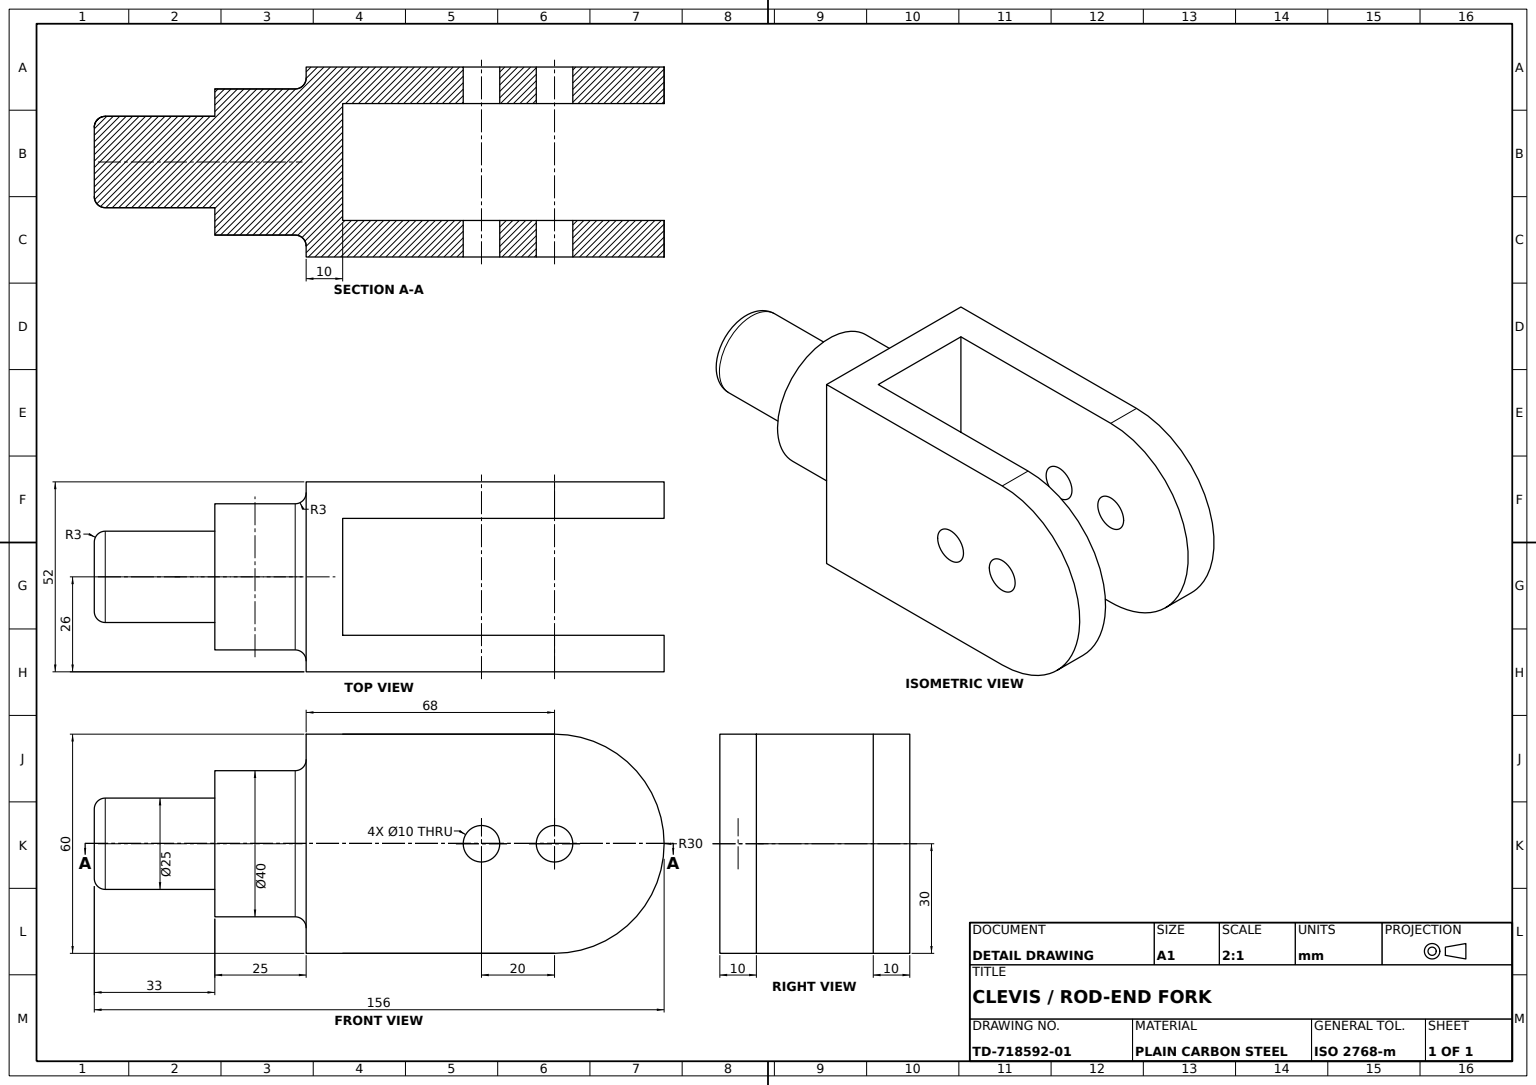
SolidWorks part; units mm, degrees
material "Plain Carbon Steel"
ref_plane "Front Plane" through (0, 0, 0) normal (0, 0, 1) x (1, 0, 0)
ref_plane "Top Plane" through (0, 0, 0) normal (0, 1, 0) x (1, 0, 0)
ref_plane "Right Plane" through (0, 0, 0) normal (1, 0, 0) x (0, 0, -1)
sketch "Front Ear Profile Sketch" plane through (0, 0, 0) normal (0, 0, 1) x (1, 0, 0)
  line L0 (0, 0) -> (68, 0)
  line L2 (68, 60) -> (0, 60)
  line L3 (0, 60) -> (0, 0)
  arc A0 (68, 60) -> (68, 0) centre (68, 30) cw
  circle A1 centre (68, 30) radius 5
  circle A2 centre (48, 30) radius 5
  dimension "D1" = 30
  dimension "D3" = 10
  dimension "D4" = 10
  dimension "D2" = 68
  dimension "D5" = 20
extrude "Front Ear Plate" add sketch "Front Ear Profile Sketch" along normal blind 10
sketch "Bridge Wall Sketch" plane through (0, 60, 0) normal (0, 1, 0) x (1, 0, 0)
  line L1 (0, 0) -> (10, 0)
  line L2 (0, 0) -> (0, 42)
  line L3 (0, 42) -> (10, 42)
  line L4 (10, 0) -> (10, 42)
  dimension "D1" = 10
  dimension "D2" = 42
extrude "Bridge Wall" add sketch "Bridge Wall Sketch" against normal blind 60
sketch "Rear Ear Profile Sketch" plane through (0, 0, -42) normal (0, 0, -1) x (-1, 0, 0)
  line L1 (-10, 60) -> (-68, 60)
  line L2 (-10, 60) -> (-10, 0)
  line L3 (-10, 0) -> (-68, 0)
  arc A0 (-68, 60) -> (-68, 0) centre (-68, 30) ccw
  circle A1 centre (-68, 30) radius 5
  circle A2 centre (-48, 30) radius 5
  dimension "D1" = 10
  dimension "D2" = 10
extrude "Rear Ear Plate" add sketch "Rear Ear Profile Sketch" against normal blind 10
sketch "Collar Sketch Ø26" plane through (0, 0, 0) normal (-1, 0, 0) x (0, 0, 1)
  line L0 (10, 0) -> (-42, 0) construction
  line L1 (-42, 0) -> (-42, 60) construction
  circle A0 centre (-16, 30) radius 20
  point P6 (-42, 30)
  dimension "D1" = 40
  dimension "D2" = 30
  dimension "D3" = 26
extrude "Shank Collar Ø26" add sketch "Collar Sketch Ø26" along normal blind 25
fillet "Collar Fillet R3" radius 3 1 edges at (0, 30, 4)
sketch "Pin Shank Sketch" plane through (-25, 0, 0) normal (-1, 0, 0) x (0, 0, 1)
  circle A0 centre (-16, 30) radius 12.5
  dimension "D1" = 25
extrude "Pin Shank" add sketch "Pin Shank Sketch" along normal blind 33
fillet "Shank End Fillet R3" radius 3 1 edges at (-58, 30, -3.5)
